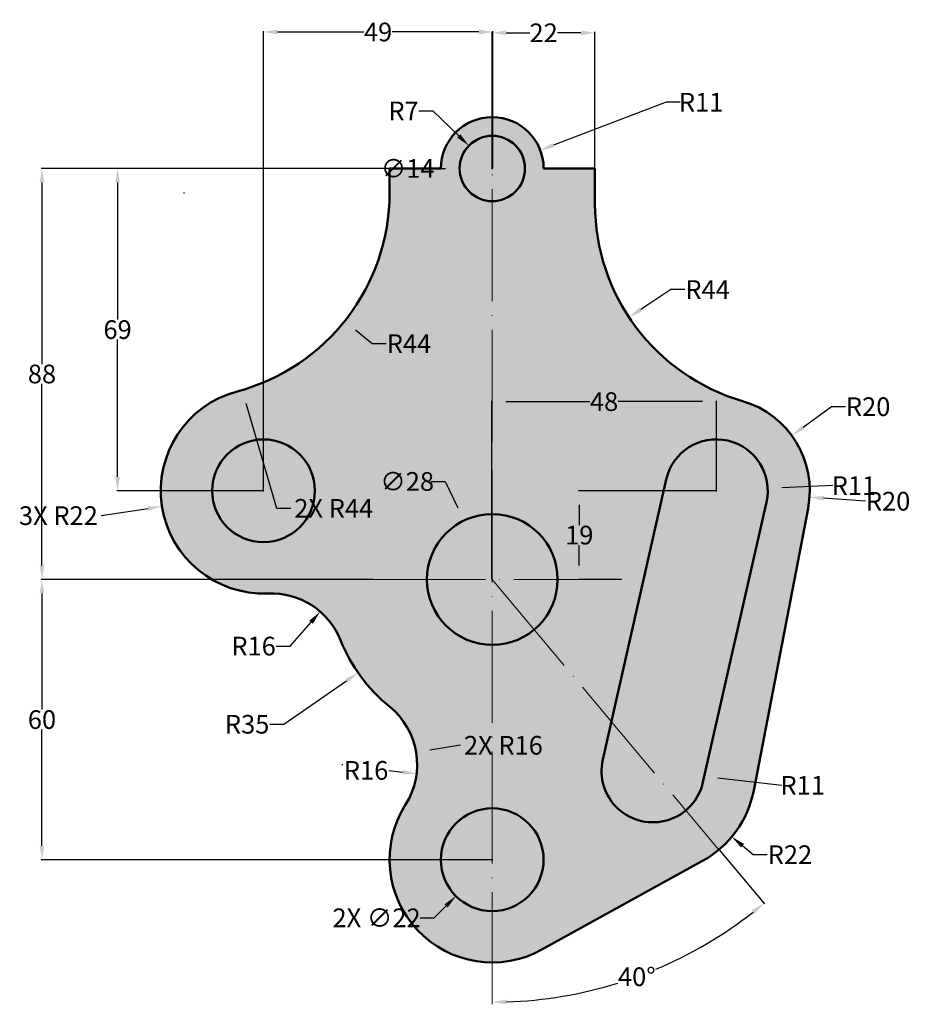
# Model space of a CAD drawing. Units: inches. Extents: x 190 to 381, y 67 to 278.
import ezdxf

# ---------------------------------------------------------------- set-up
doc = ezdxf.new("R2010")
doc.units = ezdxf.units.IN
doc.header["$MEASUREMENT"] = 0
doc.linetypes.add('ACAD_ISO04W100', pattern=[30, 24, -3, 0, -3])
for name, color, linetype, lineweight in [('M-CNTR', 18, 'ACAD_ISO04W100', 18), ('M-DIMS', 2, 'Continuous', 25), ('M-HATC', 8, 'Continuous', 18), ('M-OUTL', 7, 'Continuous', 50)]:
    doc.layers.add(name, color=color, linetype=linetype, lineweight=lineweight)
doc.styles.get("Standard").update_dxf_attribs({"font": 'arial.ttf'})
doc.dimstyles.get("Standard").update_dxf_attribs({"dimtxt": 4, "dimasz": 3, "dimexe": 0.18, "dimexo": 0.0625, "dimgap": 0.09, "dimtad": 0, "dimtih": 1, "dimtoh": 1, "dimdec": 0, "dimzin": 0, "dimdsep": 46, "dimtxsty": 'Standard', "dimcen": 0.09, "dimadec": 0, "dimazin": 0, "dimtfac": 1, "dimtdec": 0, "dimtofl": 0, "dimtmove": 0, "dimatfit": 3, "dimfxl": 1, "dimtolj": 1, "dimtzin": 0, "dimarcsym": 0})

# ---------------------------------------------------------------- blocks, each defined once
blk = doc.blocks.new('*D1')
at = {"layer": 'Defpoints', "color": 0, "transparency": 16777216}
for p in [(357.51, 238.07), (320.81, 213.81)]:
    blk.add_point(p, dxfattribs=at)
at = {"layer": 'M-DIMS', "color": 0, "lineweight": -2, "transparency": 16777216}
for p, q in [((329.77, 219.73), (323.31, 215.46)), ((332.77, 219.73), (329.77, 219.73))]:
    blk.add_line(p, q, dxfattribs=at)
at = {"layer": 'M-DIMS', "color": 0, "transparency": 16777216}
blk.add_solid([(323.03, 215.88), (323.59, 215.04), (320.81, 213.81)], dxfattribs=at)
at = {"layer": 'M-DIMS', "color": 0, "transparency": 16777216, "insert": (337.63, 219.73), "char_height": 4, "attachment_point": 5}
blk.add_mtext('\\A1;R44', dxfattribs=at)
blk = doc.blocks.new('*D2')
at = {"layer": 'Defpoints', "color": 0, "transparency": 16777216}
for p in [(301.79, 249.57), (291.51, 245.66)]:
    blk.add_point(p, dxfattribs=at)
at = {"layer": 'M-DIMS', "color": 0, "lineweight": -2, "transparency": 16777216}
for p, q in [((328.77, 259.84), (304.59, 250.64)), ((331.77, 259.84), (328.77, 259.84)), ((291.42, 245.66), (291.6, 245.66)), ((291.51, 245.57), (291.51, 245.75))]:
    blk.add_line(p, q, dxfattribs=at)
at = {"layer": 'M-DIMS', "color": 0, "transparency": 16777216}
blk.add_solid([(304.42, 251.1), (304.77, 250.17), (301.79, 249.57)], dxfattribs=at)
at = {"layer": 'M-DIMS', "color": 0, "transparency": 16777216, "insert": (336.25, 259.84), "char_height": 4, "attachment_point": 5}
blk.add_mtext('\\A1;R11', dxfattribs=at)
blk = doc.blocks.new('*D3')
at = {"layer": 'Defpoints', "color": 0, "transparency": 16777216}
for p in [(286.49, 250.54), (291.51, 245.66)]:
    blk.add_point(p, dxfattribs=at)
at = {"layer": 'M-DIMS', "color": 0, "lineweight": -2, "transparency": 16777216}
for p, q in [((275.81, 257.99), (278.81, 257.99)), ((278.81, 257.99), (284.34, 252.63)), ((291.42, 245.66), (291.6, 245.66)), ((291.51, 245.57), (291.51, 245.75))]:
    blk.add_line(p, q, dxfattribs=at)
at = {"layer": 'M-DIMS', "color": 0, "transparency": 16777216}
blk.add_solid([(284.69, 252.98), (283.99, 252.27), (286.49, 250.54)], dxfattribs=at)
at = {"layer": 'M-DIMS', "color": 0, "transparency": 16777216, "insert": (272.5, 257.99), "char_height": 4, "attachment_point": 5}
blk.add_mtext('\\A1;R7', dxfattribs=at)
blk = doc.blocks.new('*D4')
at = {"layer": 'Defpoints', "color": 0, "transparency": 16777216}
for p in [(313.51, 274.71), (291.51, 245.66), (313.51, 245.66)]:
    blk.add_point(p, dxfattribs=at)
at = {"layer": 'M-DIMS', "color": 0, "lineweight": -2, "transparency": 16777216}
for p, q in [((291.51, 245.72), (291.51, 274.89)), ((294.51, 274.71), (299.54, 274.71)), ((310.51, 274.71), (305.48, 274.71)), ((313.51, 245.72), (313.51, 274.89))]:
    blk.add_line(p, q, dxfattribs=at)
at = {"layer": 'M-DIMS', "color": 0, "transparency": 16777216}
for points in [[(294.51, 275.21), (294.51, 274.21), (291.51, 274.71)], [(310.51, 275.21), (310.51, 274.21), (313.51, 274.71)]]:
    blk.add_solid(points, dxfattribs=at)
at = {"layer": 'M-DIMS', "color": 0, "transparency": 16777216, "insert": (302.51, 274.71), "char_height": 4, "attachment_point": 5}
blk.add_mtext('\\A1;22', dxfattribs=at)
blk = doc.blocks.new('*D5')
at = {"layer": 'Defpoints', "color": 0, "transparency": 16777216}
for p in [(242.51, 274.89), (291.6, 245.66), (242.51, 176.66)]:
    blk.add_point(p, dxfattribs=at)
at = {"layer": 'M-DIMS', "color": 0, "lineweight": -2, "transparency": 16777216}
for p, q in [((242.51, 176.72), (242.51, 275.07)), ((245.51, 274.89), (264.02, 274.89)), ((288.6, 274.89), (270.09, 274.89)), ((291.6, 245.72), (291.6, 275.07))]:
    blk.add_line(p, q, dxfattribs=at)
at = {"layer": 'M-DIMS', "color": 0, "transparency": 16777216}
for points in [[(245.51, 275.39), (245.51, 274.39), (242.51, 274.89)], [(288.6, 275.39), (288.6, 274.39), (291.6, 274.89)]]:
    blk.add_solid(points, dxfattribs=at)
at = {"layer": 'M-DIMS', "color": 0, "transparency": 16777216, "insert": (267.05, 274.89), "char_height": 4, "attachment_point": 5}
blk.add_mtext('\\A1;49', dxfattribs=at)
blk = doc.blocks.new('*D6')
at = {"layer": 'Defpoints', "color": 0, "transparency": 16777216}
for p in [(225.51, 240.43), (259.85, 212.92)]:
    blk.add_point(p, dxfattribs=at)
at = {"layer": 'M-DIMS', "color": 0, "lineweight": -2, "transparency": 16777216}
for p, q in [((225.42, 240.43), (225.6, 240.43)), ((225.51, 240.34), (225.51, 240.52)), ((265.81, 208.15), (262.19, 211.05)), ((268.81, 208.15), (265.81, 208.15))]:
    blk.add_line(p, q, dxfattribs=at)
at = {"layer": 'M-DIMS', "color": 0, "transparency": 16777216}
blk.add_solid([(262.5, 211.44), (261.88, 210.66), (259.85, 212.92)], dxfattribs=at)
at = {"layer": 'M-DIMS', "color": 0, "transparency": 16777216, "insert": (273.67, 208.15), "char_height": 4, "attachment_point": 5}
blk.add_mtext('\\A1;R44', dxfattribs=at)
blk = doc.blocks.new('*D7')
at = {"layer": 'Defpoints', "color": 0, "transparency": 16777216}
for p in [(285.45, 170.28), (297.57, 145.04)]:
    blk.add_point(p, dxfattribs=at)
at = {"layer": 'M-DIMS', "color": 0, "lineweight": -2, "transparency": 16777216}
for p, q in [((278.42, 178.65), (281.42, 178.65)), ((281.42, 178.65), (284.15, 172.98)), ((291.42, 157.66), (291.6, 157.66)), ((291.51, 157.57), (291.51, 157.75))]:
    blk.add_line(p, q, dxfattribs=at)
at = {"layer": 'M-DIMS', "color": 0, "transparency": 16777216}
blk.add_solid([(284.6, 173.2), (283.69, 172.76), (285.45, 170.28)], dxfattribs=at)
at = {"layer": 'M-DIMS', "color": 0, "transparency": 16777216, "insert": (273.28, 178.65), "char_height": 4, "attachment_point": 5}
blk.add_mtext('\\A1;∅28', dxfattribs=at)
blk = doc.blocks.new('*D8')
at = {"layer": 'Defpoints', "color": 0, "transparency": 16777216}
for p in [(339.51, 195.74), (339.51, 176.66), (291.42, 157.66)]:
    blk.add_point(p, dxfattribs=at)
at = {"layer": 'M-DIMS', "color": 0, "lineweight": -2, "transparency": 16777216}
for p, q in [((291.42, 157.72), (291.42, 195.92)), ((294.42, 195.74), (312.43, 195.74)), ((336.51, 195.74), (318.5, 195.74)), ((339.51, 176.72), (339.51, 195.92))]:
    blk.add_line(p, q, dxfattribs=at)
at = {"layer": 'M-DIMS', "color": 0, "transparency": 16777216}
for points in [[(294.42, 196.24), (294.42, 195.24), (291.42, 195.74)], [(336.51, 196.24), (336.51, 195.24), (339.51, 195.74)]]:
    blk.add_solid(points, dxfattribs=at)
at = {"layer": 'M-DIMS', "color": 0, "transparency": 16777216, "insert": (315.46, 195.74), "char_height": 4, "attachment_point": 5}
blk.add_mtext('\\A1;48', dxfattribs=at)
blk = doc.blocks.new('*D9')
at = {"layer": 'Defpoints', "color": 0, "transparency": 16777216}
for p in [(339.51, 176.66), (310.14, 157.66), (319.26, 157.66)]:
    blk.add_point(p, dxfattribs=at)
at = {"layer": 'M-DIMS', "color": 0, "lineweight": -2, "transparency": 16777216}
for p, q in [((339.45, 176.66), (309.96, 176.66)), ((310.14, 173.66), (310.14, 169.29)), ((310.14, 160.66), (310.14, 165.03)), ((319.19, 157.66), (309.96, 157.66))]:
    blk.add_line(p, q, dxfattribs=at)
at = {"layer": 'M-DIMS', "color": 0, "transparency": 16777216}
for points in [[(309.64, 173.66), (310.64, 173.66), (310.14, 176.66)], [(309.64, 160.66), (310.64, 160.66), (310.14, 157.66)]]:
    blk.add_solid(points, dxfattribs=at)
at = {"layer": 'M-DIMS', "color": 0, "transparency": 16777216, "insert": (310.14, 167.16), "char_height": 4, "attachment_point": 5}
blk.add_mtext('\\A1;19', dxfattribs=at)
blk = doc.blocks.new('*D10')
at = {"layer": 'Defpoints', "color": 0, "transparency": 16777216}
for p in [(355.66, 188.45), (339.51, 176.66)]:
    blk.add_point(p, dxfattribs=at)
at = {"layer": 'M-DIMS', "color": 0, "lineweight": -2, "transparency": 16777216}
for p, q in [((364.16, 194.66), (358.08, 190.22)), ((367.16, 194.66), (364.16, 194.66)), ((339.42, 176.66), (339.6, 176.66)), ((339.51, 176.57), (339.51, 176.75))]:
    blk.add_line(p, q, dxfattribs=at)
at = {"layer": 'M-DIMS', "color": 0, "transparency": 16777216}
blk.add_solid([(357.79, 190.63), (358.38, 189.82), (355.66, 188.45)], dxfattribs=at)
at = {"layer": 'M-DIMS', "color": 0, "transparency": 16777216, "insert": (372.02, 194.66), "char_height": 4, "attachment_point": 5}
blk.add_mtext('\\A1;R20', dxfattribs=at)
blk = doc.blocks.new('*D11')
at = {"layer": 'Defpoints', "color": 0, "transparency": 16777216}
for p in [(350.5, 177.14), (339.51, 176.66)]:
    blk.add_point(p, dxfattribs=at)
at = {"layer": 'M-DIMS', "color": 0, "lineweight": -2, "transparency": 16777216}
for p, q in [((364.48, 177.75), (353.5, 177.27)), ((339.42, 176.66), (339.6, 176.66)), ((339.51, 176.57), (339.51, 176.75))]:
    blk.add_line(p, q, dxfattribs=at)
at = {"layer": 'M-DIMS', "color": 0, "transparency": 16777216}
blk.add_solid([(353.47, 177.77), (353.52, 176.77), (350.5, 177.14)], dxfattribs=at)
at = {"layer": 'M-DIMS', "color": 0, "transparency": 16777216, "insert": (368.97, 177.75), "char_height": 4, "attachment_point": 5}
blk.add_mtext('\\A1;R11', dxfattribs=at)
blk = doc.blocks.new('*D12')
at = {"layer": 'Defpoints', "color": 0, "transparency": 16777216}
for p in [(325.91, 116.66), (336.85, 115.44)]:
    blk.add_point(p, dxfattribs=at)
at = {"layer": 'M-DIMS', "color": 0, "lineweight": -2, "transparency": 16777216}
for p, q in [((325.82, 116.66), (326, 116.66)), ((325.91, 116.57), (325.91, 116.75)), ((353.52, 113.58), (339.83, 115.11))]:
    blk.add_line(p, q, dxfattribs=at)
blk.add_arc((325.91, 116.66), 11, 347.5571, 354.5787, dxfattribs=at)
at = {"layer": 'M-DIMS', "color": 0, "transparency": 16777216}
blk.add_solid([(339.88, 115.6), (339.77, 114.61), (336.85, 115.44)], dxfattribs=at)
at = {"layer": 'M-DIMS', "color": 0, "transparency": 16777216, "insert": (358, 113.58), "char_height": 4, "attachment_point": 5}
blk.add_mtext('\\A1;R11', dxfattribs=at)
blk = doc.blocks.new('*D13')
at = {"layer": 'Defpoints', "color": 0, "transparency": 16777216}
for p in [(325.91, 116.66), (342.81, 102.57)]:
    blk.add_point(p, dxfattribs=at)
at = {"layer": 'M-DIMS', "color": 0, "lineweight": -2, "transparency": 16777216}
for p, q in [((325.82, 116.66), (326, 116.66)), ((325.91, 116.57), (325.91, 116.75)), ((347.42, 98.73), (345.12, 100.65)), ((350.42, 98.73), (347.42, 98.73))]:
    blk.add_line(p, q, dxfattribs=at)
at = {"layer": 'M-DIMS', "color": 0, "transparency": 16777216}
blk.add_solid([(345.44, 101.04), (344.8, 100.27), (342.81, 102.57)], dxfattribs=at)
at = {"layer": 'M-DIMS', "color": 0, "transparency": 16777216, "insert": (355.27, 98.73), "char_height": 4, "attachment_point": 5}
blk.add_mtext('\\A1;R22', dxfattribs=at)
blk = doc.blocks.new('*D14')
at = {"layer": 'Defpoints', "color": 0, "transparency": 16777216}
for p in [(291.51, 245.66), (291.51, 157.66), (340.05, 99.8), (312.38, 69.59), (291.51, 66.74)]:
    blk.add_point(p, dxfattribs=at)
at = {"layer": 'M-DIMS', "color": 0, "lineweight": -2, "transparency": 16777216}
blk.add_line((340.09, 99.76), (349.81, 88.18), dxfattribs=at)
for start, end in [(292.7837, 308.1009), (271.8991, 287.2648)]:
    blk.add_arc((291.51, 157.66), 90.51, start, end, dxfattribs=at)
at = {"layer": 'M-DIMS', "color": 0, "transparency": 16777216}
for points in [[(347.05, 86.82), (347.68, 86.04), (349.69, 88.32)], [(294.52, 66.7), (294.5, 67.7), (291.51, 67.15)]]:
    blk.add_solid(points, dxfattribs=at)
at = {"layer": 'M-DIMS', "color": 0, "transparency": 16777216, "insert": (322.47, 72.6), "char_height": 4, "attachment_point": 5}
blk.add_mtext('\\A1;40°', dxfattribs=at)
blk = doc.blocks.new('*D15')
at = {"layer": 'Defpoints', "color": 0, "transparency": 16777216}
for p in [(269.51, 245.66), (211.25, 176.66), (242.51, 176.66)]:
    blk.add_point(p, dxfattribs=at)
at = {"layer": 'M-DIMS', "color": 0, "lineweight": -2, "transparency": 16777216}
for p, q in [((269.45, 245.66), (211.07, 245.66)), ((211.25, 242.66), (211.25, 213.29)), ((211.25, 179.66), (211.25, 209.03)), ((242.45, 176.66), (211.07, 176.66))]:
    blk.add_line(p, q, dxfattribs=at)
at = {"layer": 'M-DIMS', "color": 0, "transparency": 16777216}
for points in [[(210.75, 242.66), (211.75, 242.66), (211.25, 245.66)], [(210.75, 179.66), (211.75, 179.66), (211.25, 176.66)]]:
    blk.add_solid(points, dxfattribs=at)
at = {"layer": 'M-DIMS', "color": 0, "transparency": 16777216, "insert": (211.25, 211.16), "char_height": 4, "attachment_point": 5}
blk.add_mtext('\\A1;69', dxfattribs=at)
blk = doc.blocks.new('*D16')
at = {"layer": 'Defpoints', "color": 0, "transparency": 16777216}
for p in [(269.51, 245.66), (195.05, 157.66), (266.05, 157.66)]:
    blk.add_point(p, dxfattribs=at)
at = {"layer": 'M-DIMS', "color": 0, "lineweight": -2, "transparency": 16777216}
for p, q in [((269.45, 245.66), (194.87, 245.66)), ((195.05, 242.66), (195.05, 203.79)), ((195.05, 160.66), (195.05, 199.53)), ((265.98, 157.66), (194.87, 157.66))]:
    blk.add_line(p, q, dxfattribs=at)
at = {"layer": 'M-DIMS', "color": 0, "transparency": 16777216}
for points in [[(194.55, 242.66), (195.55, 242.66), (195.05, 245.66)], [(194.55, 160.66), (195.55, 160.66), (195.05, 157.66)]]:
    blk.add_solid(points, dxfattribs=at)
at = {"layer": 'M-DIMS', "color": 0, "transparency": 16777216, "insert": (195.05, 201.66), "char_height": 4, "attachment_point": 5}
blk.add_mtext('\\A1;88', dxfattribs=at)
blk = doc.blocks.new('*D17')
at = {"layer": 'Defpoints', "color": 0, "transparency": 16777216}
for p in [(195.05, 157.66), (266.05, 157.66), (291.51, 97.66)]:
    blk.add_point(p, dxfattribs=at)
at = {"layer": 'M-DIMS', "color": 0, "lineweight": -2, "transparency": 16777216}
for p, q in [((265.98, 157.66), (194.87, 157.66)), ((195.05, 154.66), (195.05, 129.79)), ((195.05, 100.66), (195.05, 125.53)), ((291.45, 97.66), (194.87, 97.66))]:
    blk.add_line(p, q, dxfattribs=at)
at = {"layer": 'M-DIMS', "color": 0, "transparency": 16777216}
for points in [[(194.55, 154.66), (195.55, 154.66), (195.05, 157.66)], [(194.55, 100.66), (195.55, 100.66), (195.05, 97.66)]]:
    blk.add_solid(points, dxfattribs=at)
at = {"layer": 'M-DIMS', "color": 0, "transparency": 16777216, "insert": (195.05, 127.66), "char_height": 4, "attachment_point": 5}
blk.add_mtext('\\A1;60', dxfattribs=at)
blk = doc.blocks.new('*D18')
at = {"layer": 'Defpoints', "color": 0, "transparency": 16777216}
for p in [(254.66, 150.77), (244.17, 138.69)]:
    blk.add_point(p, dxfattribs=at)
at = {"layer": 'M-DIMS', "color": 0, "lineweight": -2, "transparency": 16777216}
for p, q in [((248.25, 143.39), (252.69, 148.51)), ((245.25, 143.39), (248.25, 143.39))]:
    blk.add_line(p, q, dxfattribs=at)
at = {"layer": 'M-DIMS', "color": 0, "transparency": 16777216}
blk.add_solid([(252.31, 148.84), (253.07, 148.18), (254.66, 150.77)], dxfattribs=at)
at = {"layer": 'M-DIMS', "color": 0, "transparency": 16777216, "insert": (240.38, 143.39), "char_height": 4, "attachment_point": 5}
blk.add_mtext('\\A1;R16', dxfattribs=at)
blk = doc.blocks.new('*D19')
at = {"layer": 'Defpoints', "color": 0, "transparency": 16777216}
for p in [(291.51, 157.66), (262.76, 137.69)]:
    blk.add_point(p, dxfattribs=at)
at = {"layer": 'M-DIMS', "color": 0, "lineweight": -2, "transparency": 16777216}
for p, q in [((291.42, 157.66), (291.6, 157.66)), ((291.51, 157.57), (291.51, 157.75)), ((246.89, 126.66), (260.3, 135.98)), ((243.89, 126.66), (246.89, 126.66))]:
    blk.add_line(p, q, dxfattribs=at)
at = {"layer": 'M-DIMS', "color": 0, "transparency": 16777216}
blk.add_solid([(260.01, 136.39), (260.59, 135.57), (262.76, 137.69)], dxfattribs=at)
at = {"layer": 'M-DIMS', "color": 0, "transparency": 16777216, "insert": (239, 126.66), "char_height": 4, "attachment_point": 5}
blk.add_mtext('\\A1;R35', dxfattribs=at)
blk = doc.blocks.new('*D20')
at = {"layer": 'Defpoints', "color": 0, "transparency": 16777216}
for p in [(259.42, 118.02), (275.3, 116.04)]:
    blk.add_point(p, dxfattribs=at)
at = {"layer": 'M-DIMS', "color": 0, "lineweight": -2, "transparency": 16777216}
blk.add_line((269.35, 116.78), (272.32, 116.41), dxfattribs=at)
at = {"layer": 'M-DIMS', "color": 0, "transparency": 16777216}
blk.add_solid([(272.39, 116.9), (272.26, 115.91), (275.3, 116.04)], dxfattribs=at)
at = {"layer": 'M-DIMS', "color": 0, "transparency": 16777216, "insert": (264.48, 116.78), "char_height": 4, "attachment_point": 5}
blk.add_mtext('\\A1;R16', dxfattribs=at)
blk = doc.blocks.new('*D21')
at = {"layer": 'Defpoints', "color": 0, "transparency": 16777216}
for p in [(225.51, 240.43), (237.91, 198.22)]:
    blk.add_point(p, dxfattribs=at)
at = {"layer": 'M-DIMS', "color": 0, "lineweight": -2, "transparency": 16777216}
for p, q in [((225.42, 240.43), (225.6, 240.43)), ((225.51, 240.34), (225.51, 240.52)), ((245.35, 172.89), (238.76, 195.34)), ((248.35, 172.89), (245.35, 172.89))]:
    blk.add_line(p, q, dxfattribs=at)
at = {"layer": 'M-DIMS', "color": 0, "transparency": 16777216}
blk.add_solid([(239.24, 195.48), (238.28, 195.2), (237.91, 198.22)], dxfattribs=at)
at = {"layer": 'M-DIMS', "color": 0, "transparency": 16777216, "insert": (257.55, 172.89), "char_height": 4, "attachment_point": 5}
blk.add_mtext('\\A1;2X R44', dxfattribs=at)
blk = doc.blocks.new('*D22')
at = {"layer": 'Defpoints', "color": 0, "transparency": 16777216}
for p in [(242.51, 176.66), (220.76, 173.32)]:
    blk.add_point(p, dxfattribs=at)
at = {"layer": 'M-DIMS', "color": 0, "lineweight": -2, "transparency": 16777216}
for p, q in [((242.42, 176.66), (242.6, 176.66)), ((242.51, 176.57), (242.51, 176.75)), ((207.72, 171.33), (217.8, 172.87))]:
    blk.add_line(p, q, dxfattribs=at)
at = {"layer": 'M-DIMS', "color": 0, "transparency": 16777216}
blk.add_solid([(217.72, 173.36), (217.87, 172.38), (220.76, 173.32)], dxfattribs=at)
at = {"layer": 'M-DIMS', "color": 0, "transparency": 16777216, "insert": (198.57, 171.33), "char_height": 4, "attachment_point": 5}
blk.add_mtext('\\A1;3X R22', dxfattribs=at)
blk = doc.blocks.new('*D23')
at = {"layer": 'Defpoints', "color": 0, "transparency": 16777216}
for p in [(339.51, 176.66), (359.46, 175.26)]:
    blk.add_point(p, dxfattribs=at)
at = {"layer": 'M-DIMS', "color": 0, "lineweight": -2, "transparency": 16777216}
for p, q in [((339.42, 176.66), (339.6, 176.66)), ((339.51, 176.57), (339.51, 176.75)), ((371.43, 174.42), (362.45, 175.05))]:
    blk.add_line(p, q, dxfattribs=at)
at = {"layer": 'M-DIMS', "color": 0, "transparency": 16777216}
blk.add_solid([(362.49, 175.55), (362.42, 174.55), (359.46, 175.26)], dxfattribs=at)
at = {"layer": 'M-DIMS', "color": 0, "transparency": 16777216, "insert": (376.29, 174.42), "char_height": 4, "attachment_point": 5}
blk.add_mtext('\\A1;R20', dxfattribs=at)
blk = doc.blocks.new('*D24')
at = {"layer": 'Defpoints', "color": 0, "transparency": 16777216}
for p in [(275.21, 120.6), (259.42, 118.02)]:
    blk.add_point(p, dxfattribs=at)
at = {"layer": 'M-DIMS', "color": 0, "lineweight": -2, "transparency": 16777216}
for p, q in [((284.69, 122.16), (278.17, 121.09)), ((259.42, 117.93), (259.42, 118.11)), ((259.33, 118.02), (259.51, 118.02))]:
    blk.add_line(p, q, dxfattribs=at)
at = {"layer": 'M-DIMS', "color": 0, "transparency": 16777216}
blk.add_solid([(278.09, 121.58), (278.25, 120.6), (275.21, 120.6)], dxfattribs=at)
at = {"layer": 'M-DIMS', "color": 0, "transparency": 16777216, "insert": (293.89, 122.16), "char_height": 4, "attachment_point": 5}
blk.add_mtext('\\A1;2X R16', dxfattribs=at)
blk = doc.blocks.new('*D25')
at = {"layer": 'Defpoints', "color": 0, "transparency": 16777216}
for p in [(299.29, 105.43), (283.73, 89.88)]:
    blk.add_point(p, dxfattribs=at)
at = {"layer": 'M-DIMS', "color": 0, "lineweight": -2, "transparency": 16777216}
for p, q in [((291.42, 97.66), (291.6, 97.66)), ((291.51, 97.57), (291.51, 97.75)), ((279.06, 85.21), (281.61, 87.76)), ((276.06, 85.21), (279.06, 85.21))]:
    blk.add_line(p, q, dxfattribs=at)
at = {"layer": 'M-DIMS', "color": 0, "transparency": 16777216}
blk.add_solid([(281.26, 88.11), (281.96, 87.41), (283.73, 89.88)], dxfattribs=at)
at = {"layer": 'M-DIMS', "color": 0, "transparency": 16777216, "insert": (266.73, 85.21), "char_height": 4, "attachment_point": 5}
blk.add_mtext('\\A1;2X ∅22', dxfattribs=at)
blk = doc.blocks.new('*D26')
at = {"layer": 'Defpoints', "color": 0, "transparency": 16777216}
for p in [(284.51, 245.66), (298.51, 245.66)]:
    blk.add_point(p, dxfattribs=at)
at = {"layer": 'M-DIMS', "color": 0, "lineweight": -2, "transparency": 16777216}
for p, q in [((278.51, 245.66), (281.51, 245.66)), ((291.42, 245.66), (291.6, 245.66)), ((291.51, 245.57), (291.51, 245.75))]:
    blk.add_line(p, q, dxfattribs=at)
at = {"layer": 'M-DIMS', "color": 0, "transparency": 16777216}
blk.add_solid([(281.51, 246.16), (281.51, 245.16), (284.51, 245.66)], dxfattribs=at)
at = {"layer": 'M-DIMS', "color": 0, "transparency": 16777216, "insert": (273.39, 245.66), "char_height": 4, "attachment_point": 5}
blk.add_mtext('\\A1;∅14', dxfattribs=at)

msp = doc.modelspace()

# ---------------------------------------------------------------- hatches: boundary and pattern name
at = {"layer": 'M-HATC'}
h = msp.add_hatch(color=256, dxfattribs=at)
h.set_gradient(color1=(255, 0, 0), color2=(255, 255, 0), tint=1, name='SPHERICAL')
h.paths.add_polyline_path([(291.51, 238.66, -0.414214), (284.51, 245.66, -1), (298.51, 245.66, -0.414214), (291.51, 238.66), (291.51, 171.66, -0.414214), (305.51, 157.66, -0.221695), (300.51, 146.93), (317.03, 127.24), (328.78, 179.09, -1), (350.24, 174.23), (336.64, 114.23, -0.163898), (332.98, 108.23), (340.05, 99.8, 0.172256), (347.52, 112.5), (359.15, 172.87, 0.386724), (345.13, 195.85, -0.332972), (313.51, 238.07), (313.51, 245.66), (302.51, 245.66, 1), (280.51, 245.66), (269.51, 245.66), (269.51, 240.43, -0.339813), (236.84, 197.92, 0.897034), (243.47, 154.68, -0.318515), (259.02, 144.64, 0.128031), (269.49, 130.45, -0.3809), (272.93, 109.44, 0.591366), (291.51, 75.66), (291.51, 86.66, -0.414214), (280.51, 97.66, -0.414214), (291.51, 108.66), (291.51, 143.66, -0.414214), (277.51, 157.66, -0.414214), (291.51, 171.66)])
h.paths.add_polyline_path([(253.51, 176.66, -1), (231.51, 176.66, -1)], flags=16)
h.paths.add_polyline_path([(315.19, 119.09), (317.03, 127.24), (300.51, 146.93, -0.176327), (291.51, 143.66), (291.51, 108.66, -0.414214), (302.51, 97.66, -0.414214), (291.51, 86.66), (291.51, 75.66, 0.126821), (302.15, 78.4), (336.55, 97.4, 0.048423), (340.05, 99.8), (332.98, 108.23, -0.718364)], flags=17)
h = msp.add_hatch(color=256, dxfattribs=at)
h.set_gradient(color1=(0, 255, 0), color2=(255, 255, 0), tint=1, name='SPHERICAL')
h.paths.add_polyline_path([(298.51, 245.66, 1), (284.51, 245.66, 1)])
h = msp.add_hatch(color=256, dxfattribs=at)
h.set_gradient(color1=(0, 255, 0), color2=(255, 255, 0), tint=1, name='SPHERICAL')
h.paths.add_polyline_path([(231.51, 176.66, 1), (253.51, 176.66, 1)])
h = msp.add_hatch(color=256, dxfattribs=at)
h.set_gradient(color1=(0, 255, 0), color2=(255, 255, 0), tint=1, name='SPHERICAL')
h.paths.add_polyline_path([(350.24, 174.23, 1), (328.78, 179.09), (317.03, 127.24), (332.98, 108.23, 0.163898), (336.64, 114.23)])
h.paths.add_polyline_path([(317.03, 127.24), (315.19, 119.09, 0.718364), (332.98, 108.23)])
h = msp.add_hatch(color=256, dxfattribs=at)
h.set_gradient(color1=(0, 255, 0), color2=(255, 255, 0), tint=1, name='SPHERICAL')
h.paths.add_polyline_path([(291.51, 171.66, 0.414214), (277.51, 157.66), (291.51, 157.66)])
h.paths.add_polyline_path([(291.51, 171.66), (291.51, 157.66), (305.51, 157.66, 0.414214)])
h.paths.add_polyline_path([(291.51, 157.66), (277.51, 157.66, 0.414214), (291.51, 143.66)])
h.paths.add_polyline_path([(305.51, 157.66), (291.51, 157.66), (300.51, 146.93, 0.221695)])
h.paths.add_polyline_path([(291.51, 157.66), (291.51, 143.66, 0.176327), (300.51, 146.93)])
h = msp.add_hatch(color=256, dxfattribs=at)
h.set_gradient(color1=(0, 255, 0), color2=(255, 255, 0), tint=1, name='SPHERICAL')
h.paths.add_polyline_path([(291.51, 108.66, 0.414214), (280.51, 97.66, 0.414214), (291.51, 86.66)])
h.paths.add_polyline_path([(302.51, 97.66, 0.414214), (291.51, 108.66), (291.51, 86.66, 0.414214)])

# ---------------------------------------------------------------- linework, layer by layer
at = {"layer": 'M-CNTR'}
for p, q in [((291.51, 66.74), (291.51, 265.74)), ((266.05, 157.66), (319.26, 157.66)), ((291.51, 157.66), (340.05, 99.8))]:
    msp.add_line(p, q, dxfattribs=at)
at = {"layer": 'M-OUTL'}
for p, q in [((269.51, 245.66), (269.51, 240.43)), ((280.51, 245.66), (269.51, 245.66)), ((302.51, 245.66), (313.51, 245.66)), ((313.51, 245.66), (313.51, 238.07)), ((315.19, 119.09), (328.78, 179.09)), ((336.64, 114.23), (350.24, 174.23)), ((347.52, 112.5), (359.15, 172.87)), ((302.15, 78.4), (336.55, 97.4))]:
    msp.add_line(p, q, dxfattribs=at)
for centre, radius in [((291.51, 245.66), 7), ((242.51, 176.66), 11), ((291.51, 157.66), 14), ((291.51, 97.66), 11)]:
    msp.add_circle(centre, radius, dxfattribs=at)
for centre, radius, start, end in [((291.51, 245.66), 11, 0, 180), ((225.51, 240.43), 44, 284.9263, 0), ((357.51, 238.07), 44, 180, 253.6652), ((242.51, 176.66), 22, 104.9263, 272.499), ((339.51, 176.66), 20, 349.0945, 73.6652), ((339.51, 176.66), 11, 347.2316, 167.2316), ((244.17, 138.69), 16, 21.8292, 92.499), ((291.51, 157.66), 35, 201.8292, 231.0129), ((259.42, 118.02), 16, 327.6055, 51.0129), ((325.91, 116.66), 11, 167.2316, 347.2316), ((325.91, 116.66), 22, 298.9108, 349.0945), ((291.51, 97.66), 22, 147.6055, 298.9108)]:
    msp.add_arc(centre, radius, start, end, dxfattribs=at)

# ---------------------------------------------------------------- dimensions: what is measured, and where the dimension line sits
at = {"layer": 'M-DIMS'}
for base, p1, p2, picture, middle in [((242.51, 274.89), (291.6, 245.66), (242.51, 176.66), '*D5', (267.05, 274.89)), ((313.51, 274.71), (291.51, 245.66), (313.51, 245.66), '*D4', (302.51, 274.71)), ((339.51, 195.74), (291.42, 157.66), (339.51, 176.66), '*D8', (315.46, 195.74))]:
    dim = msp.add_linear_dim(base=base, p1=p1, p2=p2, dimstyle='Standard', override={"dimclrd": 0, "dimclre": 0, "dimclrt": 0}, dxfattribs=at)
    dim.commit()
    dim.dimension.update_dxf_attribs({"geometry": picture, "text_midpoint": middle})
for center, mpoint, override, picture, middle in [((291.51, 245.66), (301.79, 249.57), {"dimclrd": 0, "dimclre": 0, "dimclrt": 0}, '*D2', (336.25, 259.84)), ((291.51, 245.66), (286.49, 250.54), {"dimclrd": 0, "dimclre": 0, "dimclrt": 0}, '*D3', (272.5, 257.99)), ((225.51, 240.43), (259.85, 212.92), {"dimclrd": 0, "dimclre": 0, "dimclrt": 0}, '*D6', (273.67, 208.15)), ((357.51, 238.07), (320.81, 213.81), {"dimclrd": 0, "dimclre": 0, "dimclrt": 0}, '*D1', (337.63, 219.73)), ((339.51, 176.66), (355.66, 188.45), {"dimclrd": 0, "dimclre": 0, "dimclrt": 0}, '*D10', (372.02, 194.66)), ((339.51, 176.66), (350.5, 177.14), {"dimclrd": 0, "dimclre": 0, "dimclrt": 0}, '*D11', (364.48, 177.75)), ((339.51, 176.66), (359.46, 175.26), {"dimdec": 0, "dimlfac": 1, "dimrnd": 0, "dimzin": 0, "dimdsep": 46, "dimlunit": 2}, '*D23', (371.43, 174.42)), ((291.51, 157.66), (262.76, 137.69), {"dimclrd": 0, "dimclre": 0, "dimclrt": 0}, '*D19', (239, 126.66)), ((244.17, 138.69), (254.66, 150.77), {"dimclrd": 0, "dimclre": 0, "dimclrt": 0}, '*D18', (240.38, 143.39)), ((259.42, 118.02), (275.3, 116.04), {"dimclrd": 0, "dimclre": 0, "dimclrt": 0}, '*D20', (269.35, 116.78)), ((325.91, 116.66), (336.85, 115.44), {"dimclrd": 0, "dimclre": 0, "dimclrt": 0}, '*D12', (353.52, 113.58))]:
    dim = msp.add_radius_dim(center=center, mpoint=mpoint, dimstyle='Standard', override=override, dxfattribs=at)
    dim.commit()
    dim.dimension.update_dxf_attribs({"geometry": picture, "text_midpoint": middle, "dimtype": 164})
for p1, p2, override, picture, middle in [((298.51, 245.66), (284.51, 245.66), {"dimdec": 0, "dimlfac": 1, "dimrnd": 0, "dimzin": 0, "dimdsep": 46, "dimlunit": 2}, '*D26', (278.51, 245.66)), ((297.57, 145.04), (285.45, 170.28), {"dimclrd": 0, "dimclre": 0, "dimclrt": 0}, '*D7', (273.28, 178.65))]:
    dim = msp.add_diameter_dim_2p(p1=p1, p2=p2, dimstyle='Standard', override=override, dxfattribs=at)
    dim.commit()
    dim.dimension.update_dxf_attribs({"geometry": picture, "text_midpoint": middle, "dimtype": 163})
for base, p1, p2, picture, middle in [((195.05, 157.66), (269.51, 245.66), (266.05, 157.66), '*D16', (195.05, 201.66)), ((211.25, 176.66), (269.51, 245.66), (242.51, 176.66), '*D15', (211.25, 211.16)), ((310.14, 157.66), (339.51, 176.66), (319.26, 157.66), '*D9', (310.14, 167.16)), ((195.05, 157.66), (291.51, 97.66), (266.05, 157.66), '*D17', (195.05, 127.66))]:
    dim = msp.add_linear_dim(base=base, p1=p1, p2=p2, angle=90, dimstyle='Standard', override={"dimclrd": 0, "dimclre": 0, "dimclrt": 0}, dxfattribs=at)
    dim.commit()
    dim.dimension.update_dxf_attribs({"geometry": picture, "text_midpoint": middle})
dim = msp.add_angular_dim_2l(base=(312.38, 69.59), line1=((291.51, 157.66), (340.05, 99.8)), line2=((291.51, 66.74), (291.51, 245.66)), dimstyle='Standard', override={"dimclrd": 0, "dimclre": 0, "dimclrt": 0}, dxfattribs=at)
dim.commit()
dim.dimension.update_dxf_attribs({"geometry": '*D14', "text_midpoint": (322.47, 72.6)})
for center, mpoint, text, picture, middle in [((225.51, 240.43), (237.91, 198.22), '2X <>', '*D21', (257.55, 172.89)), ((242.51, 176.66), (220.76, 173.32), '3X <>', '*D22', (207.72, 171.33)), ((259.42, 118.02), (275.21, 120.6), '2X <>', '*D24', (284.69, 122.16))]:
    dim = msp.add_radius_dim(center=center, mpoint=mpoint, text=text, dimstyle='Standard', override={"dimdec": 0, "dimlfac": 1, "dimrnd": 0, "dimzin": 0, "dimdsep": 46, "dimlunit": 2}, dxfattribs=at)
    dim.commit()
    dim.dimension.update_dxf_attribs({"geometry": picture, "text_midpoint": middle, "dimtype": 164})
dim = msp.add_radius_dim(center=(325.91, 116.66), mpoint=(342.81, 102.57), dimstyle='Standard', override={"dimclrd": 0, "dimclre": 0, "dimclrt": 0}, dxfattribs=at)
dim.commit()
dim.dimension.update_dxf_attribs({"geometry": '*D13', "text_midpoint": (355.27, 98.73)})
dim = msp.add_diameter_dim_2p(p1=(299.29, 105.43), p2=(283.73, 89.88), text='2X <>', dimstyle='Standard', override={"dimdec": 0, "dimlfac": 1, "dimrnd": 0, "dimzin": 0, "dimdsep": 46, "dimlunit": 2}, dxfattribs=at)
dim.commit()
dim.dimension.update_dxf_attribs({"geometry": '*D25', "text_midpoint": (266.73, 85.21), "dimtype": 163})

doc.saveas('drawing.dxf')
